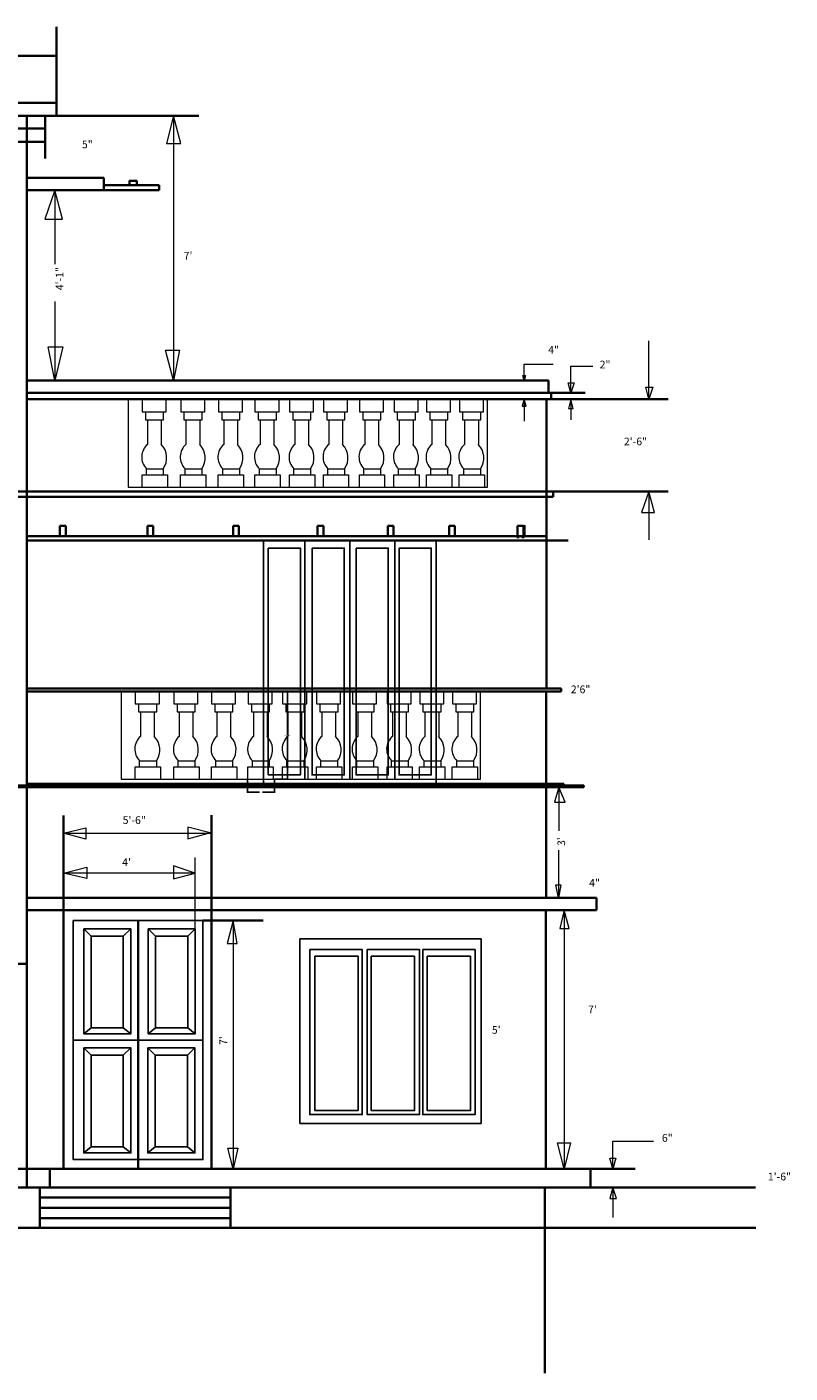
# Model space of a CAD drawing. Units: inches. Extents: x 2633 to 3277, y 1081 to 1518.
# Tile 2 of 2: x 3029 to 3277, y 1081 to 1518. Entities that reach past the tile are written whole.
import ezdxf

# ---------------------------------------------------------------- set-up
doc = ezdxf.new("R2010")
doc.units = ezdxf.units.IN
for name, color, linetype, lineweight in [('A-ANNO-DIMS', 2, 'Continuous', 18), ('A-ANNO-TEXT', 7, 'Continuous', 18), ('A-DOOR', 3, 'Continuous', 25), ('A-ELEV', 7, 'Continuous', 35), ('A-ELEV-RAIL', 8, 'Continuous', 18), ('A-GLAZ', 4, 'Continuous', 25)]:
    doc.layers.add(name, color=color, linetype=linetype, lineweight=lineweight)
doc.styles.get("Standard").update_dxf_attribs({"font": 'arial.ttf'})
doc.dimstyles.get("Standard").update_dxf_attribs({"dimtxt": 0.18, "dimasz": 0.18, "dimexe": 0.18, "dimexo": 0.0625, "dimgap": 0.09, "dimtad": 0, "dimtih": 1, "dimtoh": 1, "dimdec": 4, "dimzin": 0, "dimdsep": 46, "dimtxsty": 'Standard', "dimcen": 0.09, "dimadec": 0, "dimazin": 0, "dimtfac": 1, "dimtdec": 4, "dimtofl": 0, "dimtmove": 0, "dimatfit": 3, "dimfxl": 1, "dimtolj": 1, "dimtzin": 0, "dimarcsym": 0})

# ---------------------------------------------------------------- blocks, each defined once
blk = doc.blocks.new('BALUSTER')
for p, q in [((3063.97, 1302.32), (3063.97, 1298.28)), ((3063.97, 1298.28), (3071.78, 1298.28)), ((3065.02, 1298.28), (3065.02, 1295.72)), ((3070.93, 1295.72), (3070.93, 1298.28)), ((3071.78, 1298.28), (3071.78, 1302.32)), ((3065.02, 1295.72), (3070.93, 1295.72)), ((3065.67, 1295.72), (3065.67, 1287.7)), ((3070.14, 1295.72), (3070.14, 1287.7)), ((3063.92, 1273.87), (3063.92, 1277.87)), ((3063.92, 1277.87), (3072.14, 1277.87)), ((3065.38, 1277.87), (3065.38, 1279.8)), ((3065.38, 1279.8), (3070.8, 1279.8)), ((3070.8, 1279.8), (3070.8, 1277.87)), ((3072.14, 1277.87), (3072.14, 1273.87))]:
    blk.add_line(p, q)
for centre, radius, start, end in [((3069.2, 1283.62), 5.4, 130.7621, 224.9687), ((3065.78, 1283.36), 6.15, 324.6615, 44.8884)]:
    blk.add_arc(centre, radius, start, end)
blk = doc.blocks.new('CORBEL-B')
for p, q in [((0, 0), (0, 3.34)), ((0, 3.34), (1.89, 3.34)), ((1.89, 3.34), (1.89, 0))]:
    blk.add_line(p, q)
blk = doc.blocks.new('*D10')
at = {"layer": 'A-ANNO-DIMS', "color": 0, "lineweight": -2, "transparency": 16777216}
for p, q in [((3109.25, 1302.32), (3113.63, 1302.32)), ((3113.45, 1302.14), (3113.45, 1288.28)), ((3113.45, 1274.05), (3113.45, 1287.91)), ((3109.25, 1273.87), (3113.63, 1273.87))]:
    blk.add_line(p, q, dxfattribs=at)
at = {"layer": 'A-ANNO-DIMS', "color": 0, "transparency": 16777216}
for points in [[(3113.42, 1302.14), (3113.48, 1302.14), (3113.45, 1302.32)], [(3113.42, 1274.05), (3113.48, 1274.05), (3113.45, 1273.87)]]:
    blk.add_solid(points, dxfattribs=at)
at = {"layer": 'Defpoints', "color": 0, "transparency": 16777216}
for p in [(3109.19, 1302.32), (3113.45, 1302.32), (3109.19, 1273.87)]:
    blk.add_point(p, dxfattribs=at)
at = {"layer": 'A-ANNO-DIMS', "color": 0, "transparency": 16777216, "insert": (3113.45, 1288.09), "char_height": 0.18, "attachment_point": 5}
blk.add_mtext('\\A1;BALUSTER 28 TYP.', dxfattribs=at)
blk = doc.blocks.new('*D11')
at = {"layer": 'A-ANNO-DIMS', "color": 0, "lineweight": -2, "transparency": 16777216}
for p, q in [((3100.41, 1273.81), (3100.41, 1269.42)), ((3109.19, 1273.81), (3109.19, 1269.42)), ((3100.59, 1269.6), (3104.34, 1269.6)), ((3109.01, 1269.6), (3105.25, 1269.6))]:
    blk.add_line(p, q, dxfattribs=at)
at = {"layer": 'A-ANNO-DIMS', "color": 0, "transparency": 16777216}
for points in [[(3100.59, 1269.63), (3100.59, 1269.57), (3100.41, 1269.6)], [(3109.01, 1269.63), (3109.01, 1269.57), (3109.19, 1269.6)]]:
    blk.add_solid(points, dxfattribs=at)
at = {"layer": 'Defpoints', "color": 0, "transparency": 16777216}
for p in [(3100.41, 1273.87), (3109.19, 1273.87), (3109.19, 1269.6)]:
    blk.add_point(p, dxfattribs=at)
at = {"layer": 'A-ANNO-DIMS', "color": 0, "transparency": 16777216, "insert": (3104.8, 1269.6), "char_height": 0.18, "attachment_point": 5}
blk.add_mtext('\\A1;9 TYP.', dxfattribs=at)
blk = doc.blocks.new('*D14')
at = {"layer": 'A-ANNO-DIMS', "color": 0, "lineweight": -2, "transparency": 16777216}
for p, q in [((3190.16, 1356.11), (3190.78, 1356.11)), ((3190.6, 1355.93), (3190.6, 1354.62)), ((3190.16, 1352.76), (3190.78, 1352.76)), ((3190.6, 1352.94), (3190.6, 1354.25))]:
    blk.add_line(p, q, dxfattribs=at)
at = {"layer": 'A-ANNO-DIMS', "color": 0, "transparency": 16777216}
for points in [[(3190.57, 1355.93), (3190.63, 1355.93), (3190.6, 1356.11)], [(3190.57, 1352.94), (3190.63, 1352.94), (3190.6, 1352.76)]]:
    blk.add_solid(points, dxfattribs=at)
at = {"layer": 'Defpoints', "color": 0, "transparency": 16777216}
for p in [(3190.1, 1356.11), (3190.6, 1356.11), (3190.1, 1352.76)]:
    blk.add_point(p, dxfattribs=at)
at = {"layer": 'A-ANNO-DIMS', "color": 0, "transparency": 16777216, "insert": (3190.6, 1354.43), "char_height": 0.18, "attachment_point": 5}
blk.add_mtext('\\A1;CORBEL B 3 TYP.', dxfattribs=at)
blk = doc.blocks.new('*D15')
at = {"layer": 'A-ANNO-DIMS', "color": 0, "lineweight": -2, "transparency": 16777216}
for p, q in [((3188.21, 1352.7), (3188.21, 1352.08)), ((3188.39, 1352.26), (3188.7, 1352.26)), ((3189.92, 1352.26), (3189.62, 1352.26)), ((3190.1, 1352.7), (3190.1, 1352.08))]:
    blk.add_line(p, q, dxfattribs=at)
at = {"layer": 'A-ANNO-DIMS', "color": 0, "transparency": 16777216}
for points in [[(3188.39, 1352.29), (3188.39, 1352.23), (3188.21, 1352.26)], [(3189.92, 1352.29), (3189.92, 1352.23), (3190.1, 1352.26)]]:
    blk.add_solid(points, dxfattribs=at)
at = {"layer": 'Defpoints', "color": 0, "transparency": 16777216}
for p in [(3188.21, 1352.76), (3190.1, 1352.76), (3190.1, 1352.26)]:
    blk.add_point(p, dxfattribs=at)
at = {"layer": 'A-ANNO-DIMS', "color": 0, "transparency": 16777216, "insert": (3189.16, 1352.26), "char_height": 0.18, "attachment_point": 5}
blk.add_mtext('\\A1;2 TYP.', dxfattribs=at)

msp = doc.modelspace()

# ---------------------------------------------------------------- linework, layer by layer
at = {"layer": 'A-ANNO-DIMS'}
for p, q in [((3076.34, 1489.27), (3074.11, 1480.28)), ((3076.34, 1489.27), (3076.34, 1403.27)), ((3078.75, 1480.28), (3076.34, 1489.27)), ((3074.11, 1480.28), (3078.75, 1480.28)), ((3037.77, 1465.07), (3034.54, 1455.63)), ((3037.77, 1465.07), (3037.77, 1441.09)), ((3040.25, 1455.63), (3037.77, 1465.07)), ((3034.54, 1455.63), (3040.25, 1455.63)), ((3037.77, 1428.92), (3037.77, 1403.27)), ((3037.77, 1403.27), (3035.62, 1414.2)), ((3035.62, 1414.2), (3040.36, 1414.2)), ((3040.36, 1414.2), (3037.77, 1403.27)), ((3076.34, 1403.27), (3073.82, 1413.09)), ((3073.82, 1413.09), (3078.36, 1413.09)), ((3078.36, 1413.09), (3076.34, 1403.27)), ((3230.84, 1397.27), (3230.84, 1416.18)), ((3190.34, 1403.27), (3190.34, 1408.58)), ((3190.34, 1408.58), (3199.79, 1408.58)), ((3205.47, 1399.27), (3205.47, 1407.95)), ((3205.47, 1407.95), (3212.7, 1407.95)), ((3190.34, 1403.27), (3189.93, 1404.9)), ((3189.93, 1404.9), (3190.82, 1404.9)), ((3190.82, 1404.9), (3190.34, 1403.27)), ((3205.47, 1399.27), (3204.61, 1402.48)), ((3204.61, 1402.48), (3206.6, 1402.48)), ((3206.6, 1402.48), (3205.47, 1399.27)), ((3230.84, 1397.27), (3229.83, 1401.13)), ((3229.83, 1401.13), (3232.15, 1401.13)), ((3232.15, 1401.13), (3230.84, 1397.27)), ((3190.34, 1397.27), (3189.66, 1394.99)), ((3189.66, 1394.99), (3191.02, 1394.99)), ((3190.34, 1397.27), (3190.34, 1390.07)), ((3191.02, 1394.99), (3190.34, 1397.27)), ((3205.47, 1397.27), (3204.71, 1394.24)), ((3205.47, 1397.27), (3205.47, 1390.53)), ((3206.31, 1394.24), (3205.47, 1397.27)), ((3204.71, 1394.24), (3206.31, 1394.24)), ((3230.84, 1367.27), (3228.5, 1360.44)), ((3230.84, 1367.27), (3230.84, 1351.54)), ((3232.65, 1360.44), (3230.84, 1367.27)), ((3228.5, 1360.44), (3232.65, 1360.44)), ((3201.64, 1271.27), (3200.23, 1266.39)), ((3201.64, 1271.27), (3201.64, 1257.11)), ((3203.7, 1266.39), (3201.64, 1271.27)), ((3200.23, 1266.39), (3203.7, 1266.39)), ((3040.68, 1256.3), (3047.87, 1257.98)), ((3040.68, 1256.3), (3088.68, 1256.3)), ((3047.87, 1254.35), (3040.68, 1256.3)), ((3047.87, 1257.98), (3047.87, 1254.35)), ((3088.68, 1256.3), (3080.98, 1258.26)), ((3080.98, 1258.26), (3080.98, 1254.42)), ((3080.98, 1254.42), (3087.7, 1256.3)), ((3201.5, 1250.8), (3201.5, 1235.27)), ((3083.44, 1225.22), (3083.44, 1248.45)), ((3040.68, 1243.29), (3048.22, 1245.25)), ((3083.44, 1243.29), (3040.68, 1243.29)), ((3048.22, 1241.55), (3040.68, 1243.29)), ((3048.22, 1245.25), (3048.22, 1241.55)), ((3083.44, 1243.29), (3076.36, 1245.67)), ((3076.36, 1245.67), (3076.36, 1241.48)), ((3076.36, 1241.48), (3083.44, 1243.29)), ((3201.5, 1235.27), (3200.65, 1239.54)), ((3200.65, 1239.54), (3202.3, 1239.54)), ((3202.3, 1239.54), (3201.5, 1235.27)), ((3203.33, 1231.27), (3201.93, 1225.34)), ((3203.33, 1231.27), (3203.33, 1147.27)), ((3205.01, 1225.34), (3203.33, 1231.27)), ((3080.99, 1222.89), (3083.44, 1225.22)), ((3095.73, 1227.89), (3093.78, 1220.45)), ((3095.73, 1227.89), (3095.73, 1147.27)), ((3097.1, 1220.45), (3095.73, 1227.89)), ((3201.93, 1225.34), (3205.01, 1225.34)), ((3093.78, 1220.45), (3097.1, 1220.45)), ((3203.33, 1147.27), (3201.21, 1155.75)), ((3201.21, 1155.75), (3205.36, 1155.75)), ((3205.36, 1155.75), (3203.33, 1147.27)), ((3219.14, 1147.27), (3219.14, 1156.3)), ((3219.14, 1156.3), (3232.32, 1156.3)), ((3095.73, 1147.27), (3094.05, 1153.98)), ((3094.05, 1153.98), (3097.31, 1153.98)), ((3097.31, 1153.98), (3095.73, 1147.27)), ((3219.14, 1147.27), (3218.18, 1150.76)), ((3218.18, 1150.76), (3220.13, 1150.76)), ((3220.13, 1150.76), (3219.14, 1147.27)), ((3219.14, 1141.27), (3218.21, 1137.7)), ((3219.14, 1141.27), (3219.14, 1131.49)), ((3220.34, 1137.7), (3219.14, 1141.27)), ((3218.21, 1137.7), (3220.34, 1137.7))]:
    msp.add_line(p, q, dxfattribs=at)
at = {"layer": 'A-DOOR'}
for p, q in [((3119.07, 1351.3), (3119.07, 1273.87)), ((3148.32, 1351.3), (3148.32, 1273.87)), ((3049.64, 1222.89), (3047.19, 1225.22)), ((3060.07, 1222.89), (3062.52, 1225.22)), ((3070.56, 1222.89), (3068.11, 1225.22)), ((3043.79, 1189.1), (3085.93, 1189.1)), ((3049.64, 1193.12), (3047.19, 1191.16)), ((3060.07, 1193.12), (3062.52, 1191.16)), ((3070.56, 1193.12), (3068.11, 1191.16)), ((3080.99, 1193.12), (3083.44, 1191.16)), ((3049.64, 1184.22), (3047.19, 1186.54)), ((3060.07, 1184.22), (3062.52, 1186.54)), ((3070.46, 1184.22), (3068.01, 1186.54)), ((3080.89, 1184.22), (3083.34, 1186.54)), ((3049.64, 1154.44), (3047.19, 1152.48)), ((3060.07, 1154.44), (3062.52, 1152.48)), ((3070.46, 1154.44), (3068.01, 1152.48)), ((3080.89, 1154.44), (3083.34, 1152.48))]:
    msp.add_line(p, q, dxfattribs=at)
for points in [[(3161.7, 1351.3), (3105.59, 1351.3), (3105.59, 1272.32), (3161.7, 1272.32)], [(3133.65, 1351.3), (3133.65, 1351.3), (3133.65, 1273.87), (3133.65, 1273.87)], [(3107.19, 1348.86), (3117.63, 1348.86), (3117.63, 1275.24), (3107.19, 1275.24)], [(3121.42, 1348.86), (3131.86, 1348.86), (3131.86, 1275.24), (3121.42, 1275.24)], [(3135.73, 1348.86), (3146.16, 1348.86), (3146.16, 1275.24), (3135.73, 1275.24)], [(3149.69, 1348.86), (3160.13, 1348.86), (3160.13, 1275.24), (3149.69, 1275.24)], [(3043.79, 1227.89), (3085.93, 1227.89), (3085.93, 1150.3), (3043.79, 1150.3)], [(3047.19, 1225.22), (3062.52, 1225.22), (3062.52, 1191.16), (3047.19, 1191.16)], [(3068.11, 1225.22), (3083.44, 1225.22), (3083.44, 1191.16), (3068.11, 1191.16)], [(3049.64, 1222.89), (3060.07, 1222.89), (3060.07, 1193.12), (3049.64, 1193.12)], [(3070.56, 1222.89), (3080.99, 1222.89), (3080.99, 1193.12), (3070.56, 1193.12)], [(3047.19, 1186.54), (3062.52, 1186.54), (3062.52, 1152.48), (3047.19, 1152.48)], [(3068.01, 1186.54), (3083.34, 1186.54), (3083.34, 1152.48), (3068.01, 1152.48)], [(3049.64, 1184.22), (3060.07, 1184.22), (3060.07, 1154.44), (3049.64, 1154.44)], [(3070.46, 1184.22), (3080.89, 1184.22), (3080.89, 1154.44), (3070.46, 1154.44)]]:
    msp.add_lwpolyline(points, close=True, dxfattribs=at)
at = {"layer": 'A-ELEV'}
for p, q in [((3038.3, 1493.43), (3038.3, 1518.11)), ((2689.1, 1508.71), (3038.3, 1508.71)), ((2689.1, 1493.43), (3038.3, 1493.43)), ((3038.3, 1493.43), (3038.3, 1489.27)), ((2716.73, 1489.27), (3028.73, 1489.27)), ((3028.73, 1489.27), (3028.73, 1403.27)), ((3038.3, 1489.27), (3028.73, 1489.27)), ((3034.63, 1485.17), (3034.63, 1489.27)), ((3038.3, 1489.27), (3084.59, 1489.27)), ((2695.73, 1485.17), (3034.63, 1485.17)), ((3034.63, 1485.17), (3034.63, 1475.38)), ((2695.73, 1480.81), (3034.63, 1480.81)), ((3053.72, 1469.13), (3028.73, 1469.13)), ((3053.72, 1465.07), (3053.72, 1469.13)), ((3028.73, 1465.07), (3053.72, 1465.07)), ((3071.74, 1466.69), (3053.72, 1466.69)), ((3053.72, 1465.07), (3071.74, 1465.07)), ((3071.74, 1465.07), (3071.74, 1466.69)), ((3198.27, 1403.27), (3028.73, 1403.27)), ((3028.73, 1403.27), (3034.73, 1403.27)), ((3028.73, 1397.27), (3028.73, 1403.27)), ((3198.27, 1399.27), (3198.27, 1403.27)), ((3199.12, 1399.27), (3028.73, 1399.27)), ((3199.12, 1397.27), (3199.12, 1399.27)), ((3199.12, 1399.27), (3210.11, 1399.27)), ((3197.54, 1397.27), (3028.73, 1397.27)), ((3028.73, 1397.27), (3028.73, 1141.27)), ((3197.54, 1367.27), (3197.54, 1397.27)), ((3197.54, 1397.27), (3209.57, 1397.27)), ((3209.57, 1397.27), (3237.11, 1397.27)), ((3199.77, 1365.48), (2840.38, 1365.48)), ((3213.81, 1367.27), (2852.9, 1367.27)), ((3197.54, 1351.3), (3197.54, 1367.27)), ((3199.77, 1367.27), (3199.77, 1365.48)), ((3213.81, 1367.27), (3237.11, 1367.27)), ((3197.54, 1352.76), (3028.73, 1352.76)), ((3197.54, 1351.3), (3028.73, 1351.3)), ((3197.54, 1303.3), (3197.54, 1351.3)), ((3197.54, 1351.3), (3204.64, 1351.3)), ((3202.37, 1303.3), (3028.73, 1303.3)), ((3202.37, 1302.32), (3202.37, 1303.3)), ((3197.43, 1302.32), (3028.73, 1302.32)), ((3197.43, 1272.32), (3197.43, 1302.32)), ((3197.43, 1302.32), (3202.37, 1302.32)), ((3092.05, 1272.32), (3028.73, 1272.32)), ((3203.18, 1272.32), (3092.05, 1272.32)), ((3203.18, 1271.83), (3203.18, 1272.32)), ((3209.71, 1271.83), (2888.3, 1271.83)), ((3197.44, 1271.27), (2888.3, 1271.27)), ((3197.44, 1235.27), (3197.44, 1271.27)), ((3197.44, 1271.27), (3209.71, 1271.27)), ((3209.71, 1271.27), (3209.71, 1271.83)), ((3040.68, 1231.27), (3040.68, 1262.05)), ((3088.68, 1231.27), (3088.68, 1262.16)), ((3213.81, 1235.27), (3028.73, 1235.27)), ((3213.81, 1231.27), (3213.81, 1235.27)), ((3197.4, 1231.27), (3028.73, 1231.27)), ((3040.68, 1147.27), (3040.68, 1231.27)), ((3040.68, 1231.27), (3088.68, 1231.27)), ((3088.68, 1231.27), (3088.68, 1147.27)), ((3197.4, 1147.27), (3197.4, 1231.27)), ((3197.4, 1231.27), (3213.81, 1231.27)), ((3064.86, 1227.89), (3064.86, 1147.27)), ((3085.93, 1227.89), (3105.53, 1227.89)), ((3028.73, 1213.84), (2717.1, 1213.84)), ((2707.86, 1147.27), (3211.86, 1147.27)), ((3036.2, 1147.27), (3036.2, 1141.27)), ((3211.86, 1147.27), (3211.86, 1141.27)), ((3211.86, 1147.27), (3226.41, 1147.27)), ((2707.86, 1141.27), (3211.86, 1141.27)), ((3032.99, 1141.27), (3032.99, 1128.1)), ((3094.85, 1128.1), (3094.85, 1141.27)), ((3197.07, 1141.27), (3197.07, 1080.98)), ((3211.86, 1141.27), (3265.46, 1141.27)), ((3032.99, 1138), (3094.85, 1138)), ((3032.99, 1134.68), (3094.85, 1134.68)), ((3032.99, 1128.1), (2633.01, 1128.1)), ((3032.99, 1131.29), (3094.85, 1131.29)), ((3032.99, 1128.1), (3094.85, 1128.1)), ((3094.85, 1128.1), (3265.59, 1128.1))]:
    msp.add_line(p, q, dxfattribs=at)
msp.add_lwpolyline([(3062.03, 1466.69), (3064.44, 1466.69), (3064.44, 1468.08), (3062.03, 1468.08)], close=True, dxfattribs=at)
at = {"layer": 'A-ELEV-RAIL'}
for p, q in [((3061.65, 1397.14), (3061.65, 1368.7)), ((3178.37, 1368.7), (3178.37, 1397.14)), ((3061.65, 1368.7), (3178.37, 1368.7)), ((3059.42, 1302.32), (3059.42, 1273.87)), ((3176.14, 1273.87), (3176.14, 1302.32)), ((3059.42, 1273.87), (3176.14, 1273.87))]:
    msp.add_line(p, q, dxfattribs=at)
at = {"layer": 'A-GLAZ'}
for p, q in [((3117.38, 1222.02), (3176.35, 1222.02)), ((3117.38, 1162.02), (3117.38, 1222.02)), ((3176.35, 1222.02), (3176.35, 1162.02)), ((3176.35, 1162.02), (3117.38, 1162.02))]:
    msp.add_line(p, q, dxfattribs=at)
for points in [[(3120.67, 1218.49), (3137.73, 1218.49), (3137.73, 1164.91), (3120.67, 1164.91)], [(3122.34, 1216.31), (3136.37, 1216.31), (3136.37, 1166.23), (3122.34, 1166.23)], [(3139.32, 1218.49), (3156.37, 1218.49), (3156.37, 1164.91), (3139.32, 1164.91)], [(3140.62, 1216.31), (3154.65, 1216.31), (3154.65, 1166.23), (3140.62, 1166.23)], [(3157.36, 1218.49), (3174.41, 1218.49), (3174.41, 1164.91), (3157.36, 1164.91)], [(3158.85, 1216.31), (3172.88, 1216.31), (3172.88, 1166.23), (3158.85, 1166.23)]]:
    msp.add_lwpolyline(points, close=True, dxfattribs=at)

# ---------------------------------------------------------------- block references
at = {"layer": 'A-ELEV'}
for p in [(3039.49, 1352.76), (3067.88, 1352.76), (3095.75, 1352.76), (3123.2, 1352.76), (3146.01, 1352.76), (3165.91, 1352.76), (3188.21, 1352.76)]:
    msp.add_blockref('CORBEL-B', p, dxfattribs=at)
at = {"layer": 'A-ELEV-RAIL'}
for p in [(2.24, 94.83), (14.76, 94.83), (27.02, 94.83), (38.89, 94.83), (50.12, 94.83), (61.16, 94.83), (72.85, 94.83), (84.07, 94.83), (94.64, 94.83), (105.3, 94.83), (0, 0), (12.53, 0), (24.78, 0), (36.66, 0), (47.88, 0), (58.92, 0), (70.61, 0), (81.84, 0), (92.41, 0), (103.07, 0)]:
    msp.add_blockref('BALUSTER', p, dxfattribs=at)

# ---------------------------------------------------------------- texts
at = {"layer": 'A-ANNO-TEXT', "char_height": 2.5, "attachment_point": 1}
for s, width, insert in [('5"', 14.9487, (3046.61, 1481.21)), ("7'", 23.8672, (3079.7, 1445.06)), ('4"', 4.2831, (3198.16, 1414.52)), ('2"', 3.4677, (3214.87, 1409.73)), ('2\'-6"', 17.3568, (3222.74, 1384.74)), ('2\'6"', 12.9712, (3205.49, 1304.25)), ('5\'-6"', 9.2953, (3059.86, 1261.79)), ("4'", 6.0426, (3059.69, 1248.12)), ('4"', 5.2792, (3211.46, 1241.42)), ("7'", 20.0361, (3211.1, 1200.31)), ("5'", 7.0543, (3179.84, 1193.67)), ('6"', 7.4878, (3235.09, 1158.59)), ('1\'-6"', 12.9334, (3269.53, 1146.03))]:
    msp.add_mtext_dynamic_manual_height_columns(s, width=width, gutter_width=12.5, heights=[0], dxfattribs=dict(at, insert=insert))
at = {"layer": 'A-ANNO-TEXT', "char_height": 2.5, "attachment_point": 1, "rotation": 90}
for s, width, insert in [('4\'-1"', 18.7163, (3038.12, 1432.59)), ("3'", 10.8892, (3201.15, 1252.14)), ("7'", 2.0882, (3091.32, 1187.51))]:
    msp.add_mtext_dynamic_manual_height_columns(s, width=width, gutter_width=12.5, heights=[0], dxfattribs=dict(at, insert=insert))

# ---------------------------------------------------------------- dimensions: what is measured, and where the dimension line sits
at = {"layer": 'A-ANNO-DIMS'}
for base, p1, p2, text, picture, middle in [((3190.6, 1356.11), (3190.1, 1352.76), (3190.1, 1356.11), 'CORBEL B <> TYP.', '*D14', (3190.6, 1354.43)), ((3113.45, 1302.32), (3109.19, 1273.87), (3109.19, 1302.32), 'BALUSTER <> TYP.', '*D10', (3113.45, 1288.09))]:
    dim = msp.add_linear_dim(base=base, p1=p1, p2=p2, angle=90, text=text, dimstyle='Standard', override={"dimdec": 0, "dimlfac": 1, "dimrnd": 0, "dimzin": 0, "dimdsep": 46, "dimlunit": 2}, dxfattribs=at)
    dim.commit()
    dim.dimension.update_dxf_attribs({"geometry": picture, "text_midpoint": middle})
for base, p1, p2, picture, middle in [((3190.1, 1352.26), (3188.21, 1352.76), (3190.1, 1352.76), '*D15', (3189.16, 1352.26)), ((3109.19, 1269.6), (3100.41, 1273.87), (3109.19, 1273.87), '*D11', (3104.8, 1269.6))]:
    dim = msp.add_linear_dim(base=base, p1=p1, p2=p2, text='<> TYP.', dimstyle='Standard', override={"dimdec": 0, "dimlfac": 1, "dimrnd": 0, "dimzin": 0, "dimdsep": 46, "dimlunit": 2}, dxfattribs=at)
    dim.commit()
    dim.dimension.update_dxf_attribs({"geometry": picture, "text_midpoint": middle})

doc.saveas('drawing.dxf')
